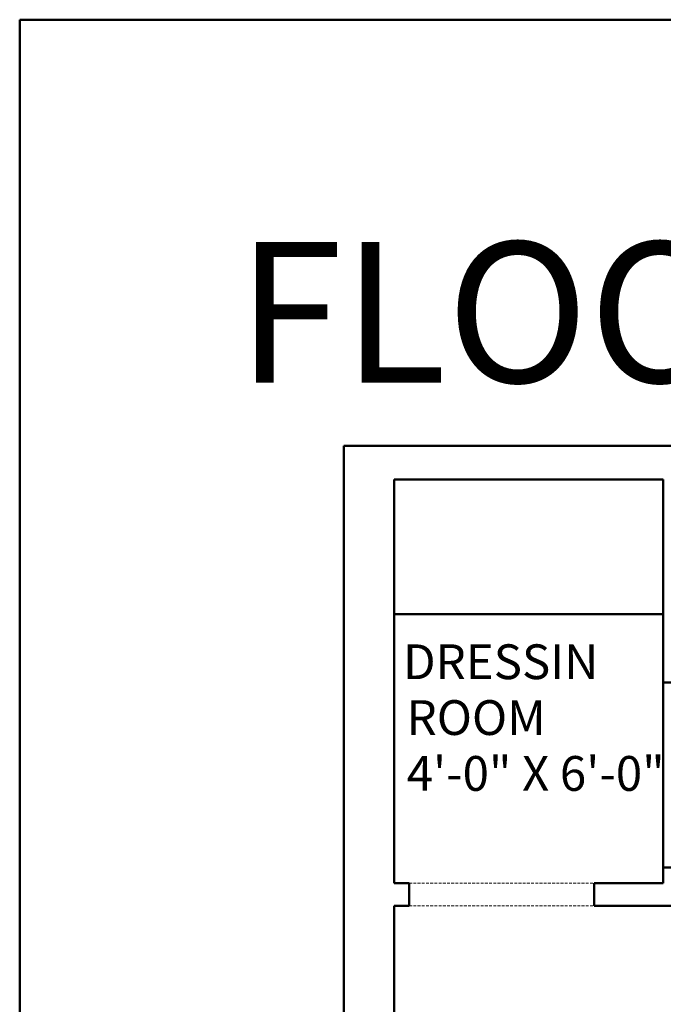
# Model space of a CAD drawing. Units: inches. Extents: x 64 to 1167, y 117 to 939.
# Tile 12 of 56: x 64 to 179, y 764 to 939. Entities that reach past the tile are written whole.
import ezdxf

# ---------------------------------------------------------------- set-up
doc = ezdxf.new("R2010")
doc.units = ezdxf.units.IN
doc.header["$MEASUREMENT"] = 0
doc.linetypes.add('DASHED', pattern=[0.75, 0.5, -0.25])
for name, color, linetype, lineweight in [('A-ANNO-TEXT', 7, 'Continuous', 25), ('A-ANNO-TTLB', 7, 'Continuous', 50), ('A-FLOR-OVHD', 8, 'DASHED', 18), ('A-WALL', 7, 'Continuous', 50)]:
    doc.layers.add(name, color=color, linetype=linetype, lineweight=lineweight)
doc.styles.get("Standard").update_dxf_attribs({"font": 'arial.ttf'})

msp = doc.modelspace()

# ---------------------------------------------------------------- linework, layer by layer
at = {"layer": 'A-ANNO-TTLB'}
msp.add_lwpolyline([(64.31, 939.22), (512.77, 939.22), (512.77, 116.55), (64.31, 116.55)], close=True, dxfattribs=at)
at = {"layer": 'A-FLOR-OVHD'}
for p, q in [((133.79, 785.2), (166.79, 785.2)), ((133.79, 781.2), (166.79, 781.2))]:
    msp.add_line(p, q, dxfattribs=at)
at = {"layer": 'A-WALL'}
for p, q in [((476.11, 863.2), (122.11, 863.2)), ((122.11, 863.2), (122.11, 155.2)), ((131.11, 857.2), (131.11, 785.2)), ((179.11, 857.2), (131.11, 857.2)), ((179.11, 857.2), (179.11, 821.03)), ((179.11, 833.2), (131.11, 833.2)), ((183.11, 821.03), (179.11, 821.03)), ((179.11, 788.04), (179.11, 821.03)), ((183.11, 788.04), (179.11, 788.04)), ((179.11, 788.04), (179.11, 785.2)), ((133.79, 785.2), (131.11, 785.2)), ((133.79, 785.2), (133.79, 781.2)), ((179.11, 785.2), (166.79, 785.2)), ((166.79, 785.2), (166.79, 781.2)), ((131.11, 781.2), (131.11, 637.2)), ((133.79, 781.2), (131.11, 781.2)), ((297.11, 781.2), (166.79, 781.2))]:
    msp.add_line(p, q, dxfattribs=at)

# ---------------------------------------------------------------- texts
at = {"layer": 'A-ANNO-TEXT'}
for s, height, p in [('FLOOR PLAN OF 3BHK', 25.0713, (102.99, 874.51)), ('DRESSIN', 6.202, (132.68, 821.61)), ('ROOM', 6.202, (133.33, 811.65)), ('4\'-0" X 6\'-0"', 6.2017, (133.33, 801.69))]:
    msp.add_text(s, height=height, dxfattribs=at).set_placement(p)

doc.saveas('drawing.dxf')
